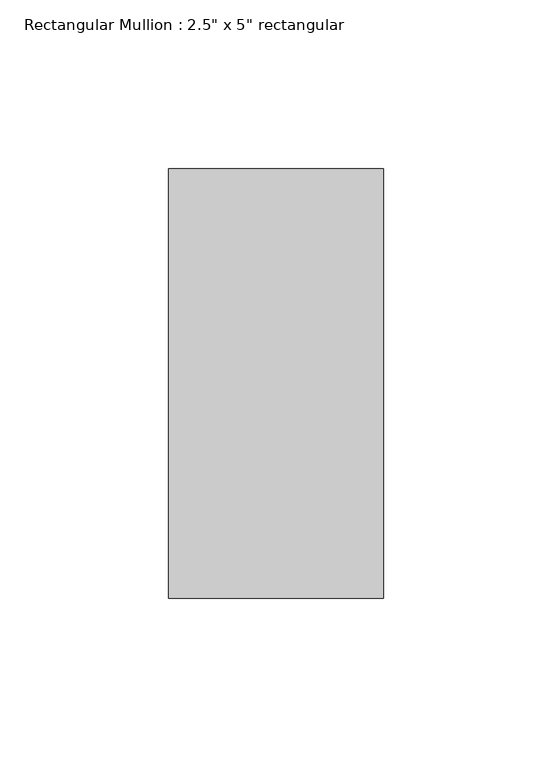
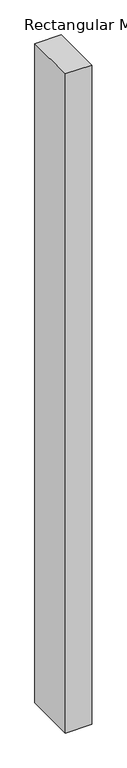
"""IFC4 building model written with IfcOpenShell, lengths in millimetres: member geometry."""

from ifc_helpers import new_model, si_unit, frame, origin, place, context, project, spatial, polyline, outline, extrude, source, transform, mapped, element, save


def member_75d123ff(model_context):
    return source(origin(), model_context, "Body", "SweptSolid", [
        extrude(outline(polyline([(0.0, 63.5), (0.0, -63.5), (-63.5, -63.5), (-63.5, 63.5), (0.0, 63.5)])), frame((0.0, 0.0, -1673.4926716), z_axis=(0.0, 0.0, 1.0), x_axis=(1.0, 0.0, 0.0)), (0.0, 0.0, 1.0), 1673.4926716),
    ])


if __name__ == "__main__":
    model = new_model("IFC4")
    model_context = context("Model", 3, world=origin())
    ifc_project = project(units=[si_unit("LENGTHUNIT", "METRE", prefix="MILLI")], contexts=[model_context])
    site = spatial("IfcSite", under=ifc_project)
    building = spatial("IfcBuilding", under=site)
    placement = place(None, origin())
    member_shape = member_75d123ff(model_context)
    element("IfcMember", 1, ObjectType="Rectangular Mullion : 2.5\" x 5\" rectangular", at=placement, inside=building, context=model_context, shape_type="MappedRepresentation", body=[
        mapped(member_shape, transform((0.0, 0.0, 0.0), x_axis=(1.0, 0.0, 0.0), y_axis=(0.0, 1.0, 0.0), z_axis=(0.0, 0.0, 1.0))),
    ])
    save(model, "model.ifc")

# Revit data of these elements
# Type "Rectangular Mullion : 2.5\" x 5\" rectangular"
#   built-in parameter 1007304 = 0.416667 (stored number, unit not read)
#   built-in parameter 1007301 = 0.104167 (stored number, unit not read)
#   built-in parameter 1007300 = 0.104167 (stored number, unit not read)
# Element 1 (IfcMember, "Rectangular Mullion : 2.5\" x 5\" rectangular")
#   Materials on its faces: "Aluminum"
# Materials
#   "Aluminum": class "Metal", colour RGB 247 247 247, transparency 0, Description = "Aluminum 6061", Cost = 0
